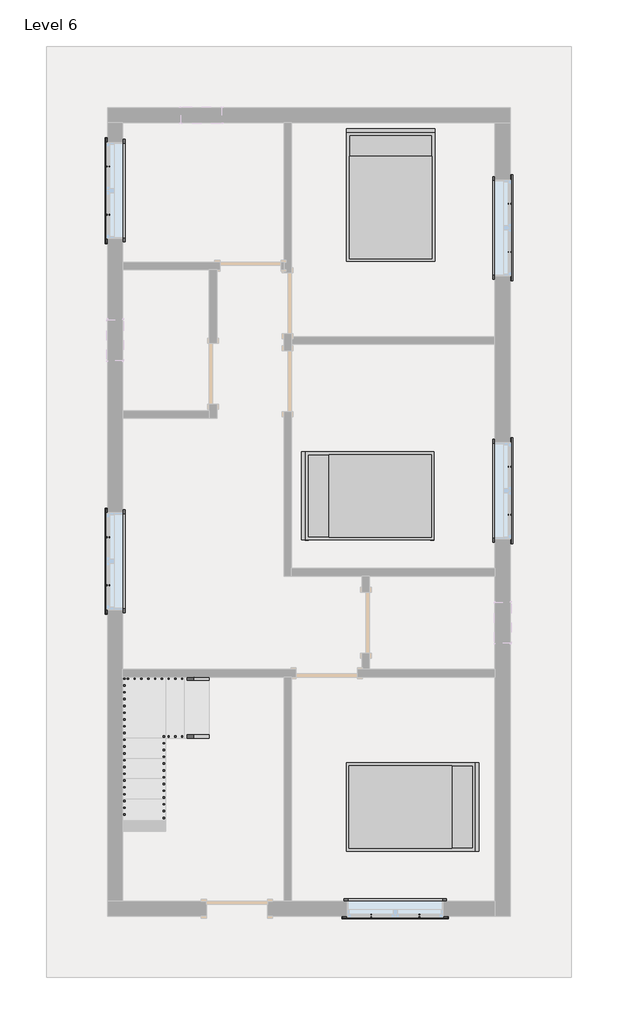
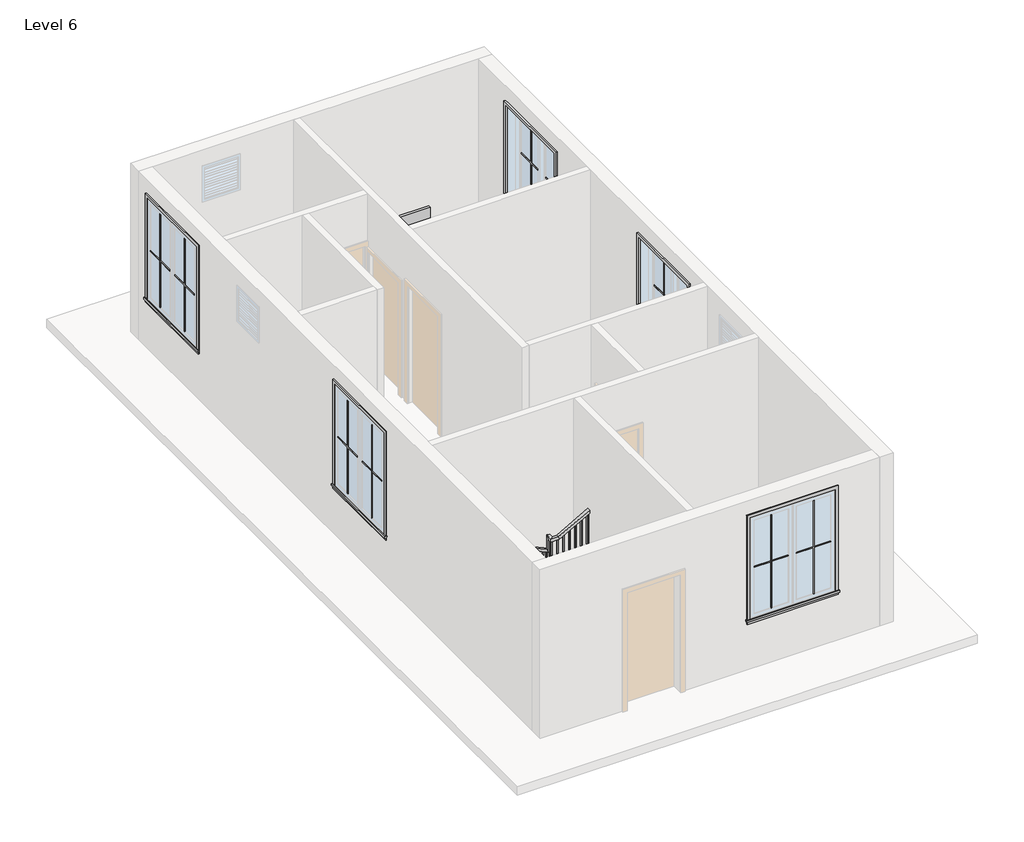
# One storey, part 2 of 2: 20 proxies, 3 furniture elements, 2 railings.
"""IFC4 building model written with IfcOpenShell, lengths in millimetres."""

from ifc_helpers import new_model, si_unit, frame, origin, place, context, project, spatial, polyline, outline, extrude, faceted_brep, transform, mapped, element, save
from components import muntin_pattern_2x2_muntin_pattern_2x2_bff912c5, muntin_pattern_2x2_muntin_pattern_2x2_c2194282, trim_window_exterior_flat_with_sill_e04b3088, trim_window_interior_flat_picture_frame_2a7685fe, bed_17739_bed_17739_15c61121

model = new_model("IFC4")

# Units and contexts
model_context = context("Model", 3, world=origin())
ifc_project = project(units=[si_unit("LENGTHUNIT", "METRE", prefix="MILLI")], contexts=[model_context])

# Site, building, storey
site = spatial("IfcSite", under=ifc_project)
building = spatial("IfcBuilding", under=site)
storey = spatial("IfcBuildingStorey", under=building, Name="Level 6", Elevation=12801.6)

# Proxies
placement = place(None, origin())
muntin_pattern_2x2_muntin_pattern_2x2_shape = muntin_pattern_2x2_muntin_pattern_2x2_bff912c5(model_context)
element("IfcBuildingElementProxy", 1, Name="Muntin Pattern_2x2 : Muntin Pattern_2x2", ObjectType="Muntin Pattern_2x2 : Muntin Pattern_2x2", at=placement, inside=storey, context=model_context, shape_type="MappedRepresentation", body=[
    mapped(muntin_pattern_2x2_muntin_pattern_2x2_shape, transform((-4261.9639285, 4584.2694249, 13785.85), x_axis=(0.0, 1.0, 0.0), y_axis=(-1.0, 0.0, 0.0), z_axis=(0.0, 0.0, 1.0))),
])
element("IfcBuildingElementProxy", 2, Name="Muntin Pattern_2x2 : Muntin Pattern_2x2", ObjectType="Muntin Pattern_2x2 : Muntin Pattern_2x2", at=placement, inside=storey, context=model_context, shape_type="MappedRepresentation", body=[
    mapped(muntin_pattern_2x2_muntin_pattern_2x2_shape, transform((1751.4860715, 4746.1944249, 13785.85), x_axis=(0.0, -1.0, 0.0), y_axis=(1.0, 0.0, 0.0), z_axis=(0.0, 0.0, 1.0))),
])
element("IfcBuildingElementProxy", 3, Name="Muntin Pattern_2x2 : Muntin Pattern_2x2", ObjectType="Muntin Pattern_2x2 : Muntin Pattern_2x2", at=placement, inside=storey, context=model_context, shape_type="MappedRepresentation", body=[
    mapped(muntin_pattern_2x2_muntin_pattern_2x2_shape, transform((-4261.9639285, -962.4555751, 13785.85), x_axis=(0.0, 1.0, 0.0), y_axis=(-1.0, 0.0, 0.0), z_axis=(0.0, 0.0, 1.0))),
])
element("IfcBuildingElementProxy", 4, Name="Muntin Pattern_2x2 : Muntin Pattern_2x2", ObjectType="Muntin Pattern_2x2 : Muntin Pattern_2x2", at=placement, inside=storey, context=model_context, shape_type="MappedRepresentation", body=[
    mapped(muntin_pattern_2x2_muntin_pattern_2x2_shape, transform((1751.4860715, 812.3694249, 13785.85), x_axis=(0.0, -1.0, 0.0), y_axis=(1.0, 0.0, 0.0), z_axis=(0.0, 0.0, 1.0))),
])
element("IfcBuildingElementProxy", 5, Name="Muntin Pattern_2x2 : Muntin Pattern_2x2", ObjectType="Muntin Pattern_2x2 : Muntin Pattern_2x2", at=placement, inside=storey, context=model_context, shape_type="MappedRepresentation", body=[
    mapped(muntin_pattern_2x2_muntin_pattern_2x2_shape, transform((397.3485715, -5907.5180751, 13785.85), x_axis=(-1.0, 0.0, 0.0), y_axis=(0.0, -1.0, 0.0), z_axis=(0.0, 0.0, 1.0))),
])
muntin_pattern_2x2_muntin_pattern_2x2_2_shape = muntin_pattern_2x2_muntin_pattern_2x2_c2194282(model_context)
element("IfcBuildingElementProxy", 6, Name="Muntin Pattern_2x2 : Muntin Pattern_2x2", ObjectType="Muntin Pattern_2x2 : Muntin Pattern_2x2", at=placement, inside=storey, context=model_context, shape_type="MappedRepresentation", body=[
    mapped(muntin_pattern_2x2_muntin_pattern_2x2_2_shape, transform((-4261.9639285, 5304.9944249, 13785.85), x_axis=(0.0, -1.0, 0.0), y_axis=(1.0, 0.0, 0.0), z_axis=(0.0, 0.0, 1.0))),
])
element("IfcBuildingElementProxy", 7, Name="Muntin Pattern_2x2 : Muntin Pattern_2x2", ObjectType="Muntin Pattern_2x2 : Muntin Pattern_2x2", at=placement, inside=storey, context=model_context, shape_type="MappedRepresentation", body=[
    mapped(muntin_pattern_2x2_muntin_pattern_2x2_2_shape, transform((1751.4860715, 4025.4694249, 13785.85), x_axis=(0.0, 1.0, 0.0), y_axis=(-1.0, 0.0, 0.0), z_axis=(0.0, 0.0, 1.0))),
])
element("IfcBuildingElementProxy", 8, Name="Muntin Pattern_2x2 : Muntin Pattern_2x2", ObjectType="Muntin Pattern_2x2 : Muntin Pattern_2x2", at=placement, inside=storey, context=model_context, shape_type="MappedRepresentation", body=[
    mapped(muntin_pattern_2x2_muntin_pattern_2x2_2_shape, transform((-4261.9639285, -241.7305751, 13785.85), x_axis=(0.0, -1.0, 0.0), y_axis=(1.0, 0.0, 0.0), z_axis=(0.0, 0.0, 1.0))),
])
element("IfcBuildingElementProxy", 9, Name="Muntin Pattern_2x2 : Muntin Pattern_2x2", ObjectType="Muntin Pattern_2x2 : Muntin Pattern_2x2", at=placement, inside=storey, context=model_context, shape_type="MappedRepresentation", body=[
    mapped(muntin_pattern_2x2_muntin_pattern_2x2_2_shape, transform((1751.4860715, 91.6444249, 13785.85), x_axis=(0.0, 1.0, 0.0), y_axis=(-1.0, 0.0, 0.0), z_axis=(0.0, 0.0, 1.0))),
])
element("IfcBuildingElementProxy", 10, Name="Muntin Pattern_2x2 : Muntin Pattern_2x2", ObjectType="Muntin Pattern_2x2 : Muntin Pattern_2x2", at=placement, inside=storey, context=model_context, shape_type="MappedRepresentation", body=[
    mapped(muntin_pattern_2x2_muntin_pattern_2x2_2_shape, transform((-323.3764285, -5907.5180751, 13785.85), x_axis=(1.0, 0.0, 0.0), y_axis=(0.0, 1.0, 0.0), z_axis=(0.0, 0.0, 1.0))),
])
trim_window_exterior_flat_with_sill_shape = trim_window_exterior_flat_with_sill_e04b3088(model_context)
element("IfcBuildingElementProxy", 11, Name="Trim-Window-Exterior-Flat : with Sill", ObjectType="Trim-Window-Exterior-Flat : with Sill", at=placement, inside=storey, context=model_context, shape_type="MappedRepresentation", body=[
    mapped(trim_window_exterior_flat_with_sill_shape, transform((-4271.4889285, 4944.6319249, 15544.8), x_axis=(0.0, -1.0, 0.0), y_axis=(0.0, 0.0, 1.0), z_axis=(-1.0, 0.0, 0.0))),
])
element("IfcBuildingElementProxy", 12, Name="Trim-Window-Exterior-Flat : with Sill", ObjectType="Trim-Window-Exterior-Flat : with Sill", at=placement, inside=storey, context=model_context, shape_type="MappedRepresentation", body=[
    mapped(trim_window_exterior_flat_with_sill_shape, transform((1761.0110715, 4385.8319249, 15544.8), x_axis=(0.0, 1.0, 0.0), y_axis=(0.0, 0.0, 1.0), z_axis=(1.0, 0.0, 0.0))),
])
element("IfcBuildingElementProxy", 13, Name="Trim-Window-Exterior-Flat : with Sill", ObjectType="Trim-Window-Exterior-Flat : with Sill", at=placement, inside=storey, context=model_context, shape_type="MappedRepresentation", body=[
    mapped(trim_window_exterior_flat_with_sill_shape, transform((-4271.4889285, -602.0930751, 15544.8), x_axis=(0.0, -1.0, 0.0), y_axis=(0.0, 0.0, 1.0), z_axis=(-1.0, 0.0, 0.0))),
])
element("IfcBuildingElementProxy", 14, Name="Trim-Window-Exterior-Flat : with Sill", ObjectType="Trim-Window-Exterior-Flat : with Sill", at=placement, inside=storey, context=model_context, shape_type="MappedRepresentation", body=[
    mapped(trim_window_exterior_flat_with_sill_shape, transform((1761.0110715, 452.0069249, 15544.8), x_axis=(0.0, 1.0, 0.0), y_axis=(0.0, 0.0, 1.0), z_axis=(1.0, 0.0, 0.0))),
])
element("IfcBuildingElementProxy", 15, Name="Trim-Window-Exterior-Flat : with Sill", ObjectType="Trim-Window-Exterior-Flat : with Sill", at=placement, inside=storey, context=model_context, shape_type="MappedRepresentation", body=[
    mapped(trim_window_exterior_flat_with_sill_shape, transform((36.9860715, -5917.0430751, 15544.8), x_axis=(1.0, 0.0, 0.0), y_axis=(0.0, 0.0, 1.0), z_axis=(0.0, -1.0, 0.0))),
])
trim_window_interior_flat_picture_frame_shape = trim_window_interior_flat_picture_frame_2a7685fe(model_context)
element("IfcBuildingElementProxy", 16, Name="Trim-Window-Interior-Flat : Picture Frame", ObjectType="Trim-Window-Interior-Flat : Picture Frame", at=placement, inside=storey, context=model_context, shape_type="MappedRepresentation", body=[
    mapped(trim_window_interior_flat_picture_frame_shape, transform((-4042.8889285, 4944.6319249, 15544.8), x_axis=(0.0, 1.0, 0.0), y_axis=(0.0, 0.0, 1.0), z_axis=(1.0, 0.0, 0.0))),
])
element("IfcBuildingElementProxy", 17, Name="Trim-Window-Interior-Flat : Picture Frame", ObjectType="Trim-Window-Interior-Flat : Picture Frame", at=placement, inside=storey, context=model_context, shape_type="MappedRepresentation", body=[
    mapped(trim_window_interior_flat_picture_frame_shape, transform((1532.4110715, 4385.8319249, 15544.8), x_axis=(0.0, -1.0, 0.0), y_axis=(0.0, 0.0, 1.0), z_axis=(-1.0, 0.0, 0.0))),
])
element("IfcBuildingElementProxy", 18, Name="Trim-Window-Interior-Flat : Picture Frame", ObjectType="Trim-Window-Interior-Flat : Picture Frame", at=placement, inside=storey, context=model_context, shape_type="MappedRepresentation", body=[
    mapped(trim_window_interior_flat_picture_frame_shape, transform((-4042.8889285, -602.0930751, 15544.8), x_axis=(0.0, 1.0, 0.0), y_axis=(0.0, 0.0, 1.0), z_axis=(1.0, 0.0, 0.0))),
])
element("IfcBuildingElementProxy", 19, Name="Trim-Window-Interior-Flat : Picture Frame", ObjectType="Trim-Window-Interior-Flat : Picture Frame", at=placement, inside=storey, context=model_context, shape_type="MappedRepresentation", body=[
    mapped(trim_window_interior_flat_picture_frame_shape, transform((1532.4110715, 452.0069249, 15544.8), x_axis=(0.0, -1.0, 0.0), y_axis=(0.0, 0.0, 1.0), z_axis=(-1.0, 0.0, 0.0))),
])
element("IfcBuildingElementProxy", 20, Name="Trim-Window-Interior-Flat : Picture Frame", ObjectType="Trim-Window-Interior-Flat : Picture Frame", at=placement, inside=storey, context=model_context, shape_type="MappedRepresentation", body=[
    mapped(trim_window_interior_flat_picture_frame_shape, transform((36.9860715, -5688.4430751, 15544.8), x_axis=(-1.0, 0.0, 0.0), y_axis=(0.0, 0.0, 1.0), z_axis=(0.0, 1.0, 0.0))),
])

# Furniture
bed_17739_bed_17739_shape = bed_17739_bed_17739_15c61121(model_context)
element("IfcFurniture", 21, ObjectType="Bed_17739 : Bed_17739", at=placement, inside=storey, context=model_context, shape_type="MappedRepresentation", body=[
    mapped(bed_17739_bed_17739_shape, transform((-29.6889285, 4852.5569249, 12801.6), x_axis=(1.0, 0.0, 0.0), y_axis=(0.0, 1.0, 0.0), z_axis=(0.0, 0.0, 1.0))),
])
element("IfcFurniture", 22, ObjectType="Bed_17739 : Bed_17739", at=placement, inside=storey, context=model_context, shape_type="MappedRepresentation", body=[
    mapped(bed_17739_bed_17739_shape, transform((-347.1889285, 375.8069249, 12801.6), x_axis=(0.0, 1.0, 0.0), y_axis=(-1.0, 0.0, 0.0), z_axis=(0.0, 0.0, 1.0))),
])
element("IfcFurniture", 23, ObjectType="Bed_17739 : Bed_17739", at=placement, inside=storey, context=model_context, shape_type="MappedRepresentation", body=[
    mapped(bed_17739_bed_17739_shape, transform((275.1110715, -4278.7430751, 12801.6), x_axis=(0.0, -1.0, 0.0), y_axis=(1.0, 0.0, 0.0), z_axis=(0.0, 0.0, 1.0))),
])

# Railings
element("IfcRailing", 24, ObjectType="Handrail - Rectangular", at=placement, inside=storey, context=model_context, shape_type="SolidModel", body=[
    faceted_brep([(-2747.4889285, -2386.4430751, 13885.3333333), (-2747.4889285, -2386.4430751, 13828.1271159), (-2747.4889285, -2335.6430751, 13828.1271159), (-2747.4889285, -2335.6430751, 13885.3333333), (-3396.0267484, -2386.4430751, 14221.1457967), (-3408.3987558, -2386.4430751, 14170.3457967), (-3408.3987558, -2335.6430751, 14170.3457967), (-3396.0267484, -2335.6430751, 14221.1457967), (-3992.0889285, -2386.4430751, 14221.1457967), (-3992.0889285, -2386.4430751, 14170.3457967), (-4042.8889285, -2335.6430751, 14170.3457967), (-4042.8889285, -2335.6430751, 14221.1457967), (-3992.0889285, -2940.1628326, 14221.1457967), (-3992.0889285, -2953.3285634, 14170.3457967), (-4042.8889285, -2953.3285634, 14170.3457967), (-4042.8889285, -2940.1628326, 14221.1457967), (-3992.0889285, -5061.9991591, 15400.1618165), (-3992.0889285, -5075.1648899, 15349.3618165), (-4042.8889285, -5075.1648899, 15349.3618165), (-4042.8889285, -5061.9991591, 15400.1618165), (-3992.0889285, -5637.6430751, 15400.1618165), (-3992.0889285, -5637.6430751, 15349.3618165), (-4042.8889285, -5688.4430751, 15349.3618165), (-4042.8889285, -5688.4430751, 15400.1618165), (-3418.001852, -5637.6430751, 15400.1618165), (-3404.8062484, -5637.6430751, 15349.3618165), (-3404.8062484, -5688.4430751, 15349.3618165), (-3418.001852, -5688.4430751, 15400.1618165), (-2793.6303845, -5637.6430751, 15748.0), (-2793.6303845, -5688.4430751, 15748.0), (-2793.6303845, -5688.4430751, 15689.8487115), (-2793.6303845, -5637.6430751, 15689.8487115)], [[[0, 1, 2, 3]], [[1, 0, 4, 5]], [[2, 1, 5, 6]], [[3, 2, 6, 7]], [[0, 3, 7, 4]], [[5, 4, 8, 9]], [[6, 5, 9, 10]], [[7, 6, 10, 11]], [[4, 7, 11, 8]], [[9, 8, 12, 13]], [[10, 9, 13, 14]], [[11, 10, 14, 15]], [[8, 11, 15, 12]], [[13, 12, 16, 17]], [[14, 13, 17, 18]], [[15, 14, 18, 19]], [[12, 15, 19, 16]], [[17, 16, 20, 21]], [[18, 17, 21, 22]], [[19, 18, 22, 23]], [[16, 19, 23, 20]], [[21, 20, 24, 25]], [[22, 21, 25, 26]], [[23, 22, 26, 27]], [[20, 23, 27, 24]], [[28, 29, 30, 31]], [[25, 24, 28, 31]], [[26, 25, 31, 30]], [[27, 26, 30, 29]], [[24, 27, 29, 28]]]),
    extrude(outline(polyline([(15692.5598207, -2788.7639285), (15681.9470401, -2807.8139285), (14664.2666667, -2807.8139285), (14664.2666667, -2788.7639285), (15692.5598207, -2788.7639285)])), frame((0.0, -5672.5680751, 0.0), z_axis=(0.0, 1.0, 0.0), x_axis=(0.0, 0.0, 1.0)), (0.0, 0.0, 1.0), 19.05),
    extrude(outline(polyline([(15635.9583242, -2890.3639285), (15625.3455436, -2909.4139285), (14664.2666667, -2909.4139285), (14664.2666667, -2890.3639285), (15635.9583242, -2890.3639285)])), frame((0.0, -5672.5680751, 0.0), z_axis=(0.0, 1.0, 0.0), x_axis=(0.0, 0.0, 1.0)), (0.0, 0.0, 1.0), 19.05),
    extrude(outline(polyline([(15579.3568277, -2991.9639285), (15568.7440471, -3011.0139285), (14664.2666667, -3011.0139285), (14664.2666667, -2991.9639285), (15579.3568277, -2991.9639285)])), frame((0.0, -5672.5680751, 0.0), z_axis=(0.0, 1.0, 0.0), x_axis=(0.0, 0.0, 1.0)), (0.0, 0.0, 1.0), 19.05),
    extrude(outline(polyline([(15522.7553312, -3093.5639285), (15512.1425506, -3112.6139285), (14664.2666667, -3112.6139285), (14664.2666667, -3093.5639285), (15522.7553312, -3093.5639285)])), frame((0.0, -5672.5680751, 0.0), z_axis=(0.0, 1.0, 0.0), x_axis=(0.0, 0.0, 1.0)), (0.0, 0.0, 1.0), 19.05),
    extrude(outline(polyline([(15466.1538346, -3195.1639285), (15455.5410541, -3214.2139285), (14494.9333333, -3214.2139285), (14494.9333333, -3195.1639285), (15466.1538346, -3195.1639285)])), frame((0.0, -5672.5680751, 0.0), z_axis=(0.0, 1.0, 0.0), x_axis=(0.0, 0.0, 1.0)), (0.0, 0.0, 1.0), 19.05),
    extrude(outline(polyline([(15409.5523381, -3296.7639285), (15398.9395575, -3315.8139285), (14494.9333333, -3315.8139285), (14494.9333333, -3296.7639285), (15409.5523381, -3296.7639285)])), frame((0.0, -5672.5680751, 0.0), z_axis=(0.0, 1.0, 0.0), x_axis=(0.0, 0.0, 1.0)), (0.0, 0.0, 1.0), 19.05),
    extrude(outline(polyline([(15352.9508416, -3398.3639285), (15342.338061, -3417.4139285), (14325.6, -3417.4139285), (14325.6, -3398.3639285), (15352.9508416, -3398.3639285)])), frame((0.0, -5672.5680751, 0.0), z_axis=(0.0, 1.0, 0.0), x_axis=(0.0, 0.0, 1.0)), (0.0, 0.0, 1.0), 19.05),
    extrude(outline(polyline([(-3519.0139285, -5672.5680751), (-3519.0139285, -5653.5180751), (-3499.9639285, -5653.5180751), (-3499.9639285, -5672.5680751), (-3519.0139285, -5672.5680751)])), frame((0.0, 0.0, 14325.6), z_axis=(0.0, 0.0, 1.0), x_axis=(1.0, 0.0, 0.0)), (0.0, 0.0, 1.0), 1023.7618165),
    extrude(outline(polyline([(-3620.6139285, -5672.5680751), (-3620.6139285, -5653.5180751), (-3601.5639285, -5653.5180751), (-3601.5639285, -5672.5680751), (-3620.6139285, -5672.5680751)])), frame((0.0, 0.0, 14325.6), z_axis=(0.0, 0.0, 1.0), x_axis=(1.0, 0.0, 0.0)), (0.0, 0.0, 1.0), 1023.7618165),
    extrude(outline(polyline([(-3722.2139285, -5672.5680751), (-3722.2139285, -5653.5180751), (-3703.1639285, -5653.5180751), (-3703.1639285, -5672.5680751), (-3722.2139285, -5672.5680751)])), frame((0.0, 0.0, 14325.6), z_axis=(0.0, 0.0, 1.0), x_axis=(1.0, 0.0, 0.0)), (0.0, 0.0, 1.0), 1023.7618165),
    extrude(outline(polyline([(-3823.8139285, -5672.5680751), (-3823.8139285, -5653.5180751), (-3804.7639285, -5653.5180751), (-3804.7639285, -5672.5680751), (-3823.8139285, -5672.5680751)])), frame((0.0, 0.0, 14325.6), z_axis=(0.0, 0.0, 1.0), x_axis=(1.0, 0.0, 0.0)), (0.0, 0.0, 1.0), 1023.7618165),
    extrude(outline(polyline([(-3925.4139285, -5672.5680751), (-3925.4139285, -5653.5180751), (-3906.3639285, -5653.5180751), (-3906.3639285, -5672.5680751), (-3925.4139285, -5672.5680751)])), frame((0.0, 0.0, 14325.6), z_axis=(0.0, 0.0, 1.0), x_axis=(1.0, 0.0, 0.0)), (0.0, 0.0, 1.0), 1023.7618165),
    extrude(outline(polyline([(-4027.0139285, -5602.7180751), (-4007.9639285, -5602.7180751), (-4007.9639285, -5621.7680751), (-4027.0139285, -5621.7680751), (-4027.0139285, -5602.7180751)])), frame((0.0, 0.0, 14325.6), z_axis=(0.0, 0.0, 1.0), x_axis=(1.0, 0.0, 0.0)), (0.0, 0.0, 1.0), 1023.7618165),
    extrude(outline(polyline([(-4027.0139285, -5501.1180751), (-4007.9639285, -5501.1180751), (-4007.9639285, -5520.1680751), (-4027.0139285, -5520.1680751), (-4027.0139285, -5501.1180751)])), frame((0.0, 0.0, 14325.6), z_axis=(0.0, 0.0, 1.0), x_axis=(1.0, 0.0, 0.0)), (0.0, 0.0, 1.0), 1023.7618165),
    extrude(outline(polyline([(-4027.0139285, -5399.5180751), (-4007.9639285, -5399.5180751), (-4007.9639285, -5418.5680751), (-4027.0139285, -5418.5680751), (-4027.0139285, -5399.5180751)])), frame((0.0, 0.0, 14325.6), z_axis=(0.0, 0.0, 1.0), x_axis=(1.0, 0.0, 0.0)), (0.0, 0.0, 1.0), 1023.7618165),
    extrude(outline(polyline([(-4027.0139285, -5297.9180751), (-4007.9639285, -5297.9180751), (-4007.9639285, -5316.9680751), (-4027.0139285, -5316.9680751), (-4027.0139285, -5297.9180751)])), frame((0.0, 0.0, 14325.6), z_axis=(0.0, 0.0, 1.0), x_axis=(1.0, 0.0, 0.0)), (0.0, 0.0, 1.0), 1023.7618165),
    extrude(outline(polyline([(-4027.0139285, -5196.3180751), (-4007.9639285, -5196.3180751), (-4007.9639285, -5215.3680751), (-4027.0139285, -5215.3680751), (-4027.0139285, -5196.3180751)])), frame((0.0, 0.0, 14325.6), z_axis=(0.0, 0.0, 1.0), x_axis=(1.0, 0.0, 0.0)), (0.0, 0.0, 1.0), 1023.7618165),
    extrude(outline(polyline([(-4027.0139285, -5094.7180751), (-4007.9639285, -5094.7180751), (-4007.9639285, -5113.7680751), (-4027.0139285, -5113.7680751), (-4027.0139285, -5094.7180751)])), frame((0.0, 0.0, 14325.6), z_axis=(0.0, 0.0, 1.0), x_axis=(1.0, 0.0, 0.0)), (0.0, 0.0, 1.0), 1023.7618165),
    extrude(outline(polyline([(-5012.1680751, 15314.3571119), (-4993.1180751, 15303.7718208), (-4993.1180751, 14325.6), (-5012.1680751, 14325.6), (-5012.1680751, 15314.3571119)])), frame((-4027.0139285, 0.0, 0.0), z_axis=(1.0, 0.0, 0.0), x_axis=(0.0, 1.0, 0.0)), (0.0, 0.0, 1.0), 19.05),
    extrude(outline(polyline([(-4910.5680751, 15257.9022261), (-4891.5180751, 15247.316935), (-4891.5180751, 14325.6), (-4910.5680751, 14325.6), (-4910.5680751, 15257.9022261)])), frame((-4027.0139285, 0.0, 0.0), z_axis=(1.0, 0.0, 0.0), x_axis=(0.0, 1.0, 0.0)), (0.0, 0.0, 1.0), 19.05),
    extrude(outline(polyline([(-4808.9680751, 15201.4473402), (-4789.9180751, 15190.8620491), (-4789.9180751, 14325.6), (-4808.9680751, 14325.6), (-4808.9680751, 15201.4473402)])), frame((-4027.0139285, 0.0, 0.0), z_axis=(1.0, 0.0, 0.0), x_axis=(0.0, 1.0, 0.0)), (0.0, 0.0, 1.0), 19.05),
    extrude(outline(polyline([(-4707.3680751, 15144.8358332), (-4688.3180751, 15134.2505421), (-4688.3180751, 14156.2666667), (-4707.3680751, 14156.2666667), (-4707.3680751, 15144.8358332)])), frame((-4027.0139285, 0.0, 0.0), z_axis=(1.0, 0.0, 0.0), x_axis=(0.0, 1.0, 0.0)), (0.0, 0.0, 1.0), 19.05),
    extrude(outline(polyline([(-4605.7680751, 15088.3809474), (-4586.7180751, 15077.7956563), (-4586.7180751, 14156.2666667), (-4605.7680751, 14156.2666667), (-4605.7680751, 15088.3809474)])), frame((-4027.0139285, 0.0, 0.0), z_axis=(1.0, 0.0, 0.0), x_axis=(0.0, 1.0, 0.0)), (0.0, 0.0, 1.0), 19.05),
    extrude(outline(polyline([(-4504.1680751, 15031.9260615), (-4485.1180751, 15021.3407704), (-4485.1180751, 14156.2666667), (-4504.1680751, 14156.2666667), (-4504.1680751, 15031.9260615)])), frame((-4027.0139285, 0.0, 0.0), z_axis=(1.0, 0.0, 0.0), x_axis=(0.0, 1.0, 0.0)), (0.0, 0.0, 1.0), 19.05),
    extrude(outline(polyline([(-4402.5680751, 14975.5024999), (-4383.5180751, 14964.9172088), (-4383.5180751, 13986.9333333), (-4402.5680751, 13986.9333333), (-4402.5680751, 14975.5024999)])), frame((-4027.0139285, 0.0, 0.0), z_axis=(1.0, 0.0, 0.0), x_axis=(0.0, 1.0, 0.0)), (0.0, 0.0, 1.0), 19.05),
    extrude(outline(polyline([(-4300.9680751, 14919.047614), (-4281.9180751, 14908.4623229), (-4281.9180751, 13986.9333333), (-4300.9680751, 13986.9333333), (-4300.9680751, 14919.047614)])), frame((-4027.0139285, 0.0, 0.0), z_axis=(1.0, 0.0, 0.0), x_axis=(0.0, 1.0, 0.0)), (0.0, 0.0, 1.0), 19.05),
    extrude(outline(polyline([(-4199.3680751, 14862.5927282), (-4180.3180751, 14852.0074371), (-4180.3180751, 13986.9333333), (-4199.3680751, 13986.9333333), (-4199.3680751, 14862.5927282)])), frame((-4027.0139285, 0.0, 0.0), z_axis=(1.0, 0.0, 0.0), x_axis=(0.0, 1.0, 0.0)), (0.0, 0.0, 1.0), 19.05),
    extrude(outline(polyline([(-4097.7680751, 14806.1691666), (-4078.7180751, 14795.5838755), (-4078.7180751, 13817.6), (-4097.7680751, 13817.6), (-4097.7680751, 14806.1691666)])), frame((-4027.0139285, 0.0, 0.0), z_axis=(1.0, 0.0, 0.0), x_axis=(0.0, 1.0, 0.0)), (0.0, 0.0, 1.0), 19.05),
    extrude(outline(polyline([(-3996.1680751, 14749.7142807), (-3977.1180751, 14739.1289896), (-3977.1180751, 13817.6), (-3996.1680751, 13817.6), (-3996.1680751, 14749.7142807)])), frame((-4027.0139285, 0.0, 0.0), z_axis=(1.0, 0.0, 0.0), x_axis=(0.0, 1.0, 0.0)), (0.0, 0.0, 1.0), 19.05),
    extrude(outline(polyline([(-3894.5680751, 14693.2593949), (-3875.5180751, 14682.6741038), (-3875.5180751, 13817.6), (-3894.5680751, 13817.6), (-3894.5680751, 14693.2593949)])), frame((-4027.0139285, 0.0, 0.0), z_axis=(1.0, 0.0, 0.0), x_axis=(0.0, 1.0, 0.0)), (0.0, 0.0, 1.0), 19.05),
    extrude(outline(polyline([(-3792.9680751, 14636.8358332), (-3773.9180751, 14626.2505421), (-3773.9180751, 13648.2666667), (-3792.9680751, 13648.2666667), (-3792.9680751, 14636.8358332)])), frame((-4027.0139285, 0.0, 0.0), z_axis=(1.0, 0.0, 0.0), x_axis=(0.0, 1.0, 0.0)), (0.0, 0.0, 1.0), 19.05),
    extrude(outline(polyline([(-3691.3680751, 14580.3809474), (-3672.3180751, 14569.7956563), (-3672.3180751, 13648.2666667), (-3691.3680751, 13648.2666667), (-3691.3680751, 14580.3809474)])), frame((-4027.0139285, 0.0, 0.0), z_axis=(1.0, 0.0, 0.0), x_axis=(0.0, 1.0, 0.0)), (0.0, 0.0, 1.0), 19.05),
    extrude(outline(polyline([(-3589.7680751, 14523.9260615), (-3570.7180751, 14513.3407704), (-3570.7180751, 13648.2666667), (-3589.7680751, 13648.2666667), (-3589.7680751, 14523.9260615)])), frame((-4027.0139285, 0.0, 0.0), z_axis=(1.0, 0.0, 0.0), x_axis=(0.0, 1.0, 0.0)), (0.0, 0.0, 1.0), 19.05),
    extrude(outline(polyline([(-3488.1680751, 14467.5024999), (-3469.1180751, 14456.9172088), (-3469.1180751, 13478.9333333), (-3488.1680751, 13478.9333333), (-3488.1680751, 14467.5024999)])), frame((-4027.0139285, 0.0, 0.0), z_axis=(1.0, 0.0, 0.0), x_axis=(0.0, 1.0, 0.0)), (0.0, 0.0, 1.0), 19.05),
    extrude(outline(polyline([(-3386.5680751, 14411.047614), (-3367.5180751, 14400.4623229), (-3367.5180751, 13478.9333333), (-3386.5680751, 13478.9333333), (-3386.5680751, 14411.047614)])), frame((-4027.0139285, 0.0, 0.0), z_axis=(1.0, 0.0, 0.0), x_axis=(0.0, 1.0, 0.0)), (0.0, 0.0, 1.0), 19.05),
    extrude(outline(polyline([(-3284.9680751, 14354.5927282), (-3265.9180751, 14344.0074371), (-3265.9180751, 13478.9333333), (-3284.9680751, 13478.9333333), (-3284.9680751, 14354.5927282)])), frame((-4027.0139285, 0.0, 0.0), z_axis=(1.0, 0.0, 0.0), x_axis=(0.0, 1.0, 0.0)), (0.0, 0.0, 1.0), 19.05),
    extrude(outline(polyline([(-3183.3680751, 14298.1691666), (-3164.3180751, 14287.5838755), (-3164.3180751, 13309.6), (-3183.3680751, 13309.6), (-3183.3680751, 14298.1691666)])), frame((-4027.0139285, 0.0, 0.0), z_axis=(1.0, 0.0, 0.0), x_axis=(0.0, 1.0, 0.0)), (0.0, 0.0, 1.0), 19.05),
    extrude(outline(polyline([(-3081.7680751, 14241.7142807), (-3062.7180751, 14231.1289896), (-3062.7180751, 13309.6), (-3081.7680751, 13309.6), (-3081.7680751, 14241.7142807)])), frame((-4027.0139285, 0.0, 0.0), z_axis=(1.0, 0.0, 0.0), x_axis=(0.0, 1.0, 0.0)), (0.0, 0.0, 1.0), 19.05),
    extrude(outline(polyline([(-2980.1680751, 14185.2593949), (-2961.1180751, 14174.6741038), (-2961.1180751, 13309.6), (-2980.1680751, 13309.6), (-2980.1680751, 14185.2593949)])), frame((-4027.0139285, 0.0, 0.0), z_axis=(1.0, 0.0, 0.0), x_axis=(0.0, 1.0, 0.0)), (0.0, 0.0, 1.0), 19.05),
    extrude(outline(polyline([(-4027.0139285, -2859.5180751), (-4007.9639285, -2859.5180751), (-4007.9639285, -2878.5680751), (-4027.0139285, -2878.5680751), (-4027.0139285, -2859.5180751)])), frame((0.0, 0.0, 13309.6), z_axis=(0.0, 0.0, 1.0), x_axis=(1.0, 0.0, 0.0)), (0.0, 0.0, 1.0), 860.7457967),
    extrude(outline(polyline([(-4027.0139285, -2757.9180751), (-4007.9639285, -2757.9180751), (-4007.9639285, -2776.9680751), (-4027.0139285, -2776.9680751), (-4027.0139285, -2757.9180751)])), frame((0.0, 0.0, 13309.6), z_axis=(0.0, 0.0, 1.0), x_axis=(1.0, 0.0, 0.0)), (0.0, 0.0, 1.0), 860.7457967),
    extrude(outline(polyline([(-4027.0139285, -2656.3180751), (-4007.9639285, -2656.3180751), (-4007.9639285, -2675.3680751), (-4027.0139285, -2675.3680751), (-4027.0139285, -2656.3180751)])), frame((0.0, 0.0, 13309.6), z_axis=(0.0, 0.0, 1.0), x_axis=(1.0, 0.0, 0.0)), (0.0, 0.0, 1.0), 860.7457967),
    extrude(outline(polyline([(-4027.0139285, -2554.7180751), (-4007.9639285, -2554.7180751), (-4007.9639285, -2573.7680751), (-4027.0139285, -2573.7680751), (-4027.0139285, -2554.7180751)])), frame((0.0, 0.0, 13309.6), z_axis=(0.0, 0.0, 1.0), x_axis=(1.0, 0.0, 0.0)), (0.0, 0.0, 1.0), 860.7457967),
    extrude(outline(polyline([(-4027.0139285, -2453.1180751), (-4007.9639285, -2453.1180751), (-4007.9639285, -2472.1680751), (-4027.0139285, -2472.1680751), (-4027.0139285, -2453.1180751)])), frame((0.0, 0.0, 13309.6), z_axis=(0.0, 0.0, 1.0), x_axis=(1.0, 0.0, 0.0)), (0.0, 0.0, 1.0), 860.7457967),
    extrude(outline(polyline([(-3957.1639285, -2351.5180751), (-3957.1639285, -2370.5680751), (-3976.2139285, -2370.5680751), (-3976.2139285, -2351.5180751), (-3957.1639285, -2351.5180751)])), frame((0.0, 0.0, 13309.6), z_axis=(0.0, 0.0, 1.0), x_axis=(1.0, 0.0, 0.0)), (0.0, 0.0, 1.0), 860.7457967),
    extrude(outline(polyline([(-3855.5639285, -2351.5180751), (-3855.5639285, -2370.5680751), (-3874.6139285, -2370.5680751), (-3874.6139285, -2351.5180751), (-3855.5639285, -2351.5180751)])), frame((0.0, 0.0, 13309.6), z_axis=(0.0, 0.0, 1.0), x_axis=(1.0, 0.0, 0.0)), (0.0, 0.0, 1.0), 860.7457967),
    extrude(outline(polyline([(-3753.9639285, -2351.5180751), (-3753.9639285, -2370.5680751), (-3773.0139285, -2370.5680751), (-3773.0139285, -2351.5180751), (-3753.9639285, -2351.5180751)])), frame((0.0, 0.0, 13309.6), z_axis=(0.0, 0.0, 1.0), x_axis=(1.0, 0.0, 0.0)), (0.0, 0.0, 1.0), 860.7457967),
    extrude(outline(polyline([(-3652.3639285, -2351.5180751), (-3652.3639285, -2370.5680751), (-3671.4139285, -2370.5680751), (-3671.4139285, -2351.5180751), (-3652.3639285, -2351.5180751)])), frame((0.0, 0.0, 13309.6), z_axis=(0.0, 0.0, 1.0), x_axis=(1.0, 0.0, 0.0)), (0.0, 0.0, 1.0), 860.7457967),
    extrude(outline(polyline([(-3550.7639285, -2351.5180751), (-3550.7639285, -2370.5680751), (-3569.8139285, -2370.5680751), (-3569.8139285, -2351.5180751), (-3550.7639285, -2351.5180751)])), frame((0.0, 0.0, 13309.6), z_axis=(0.0, 0.0, 1.0), x_axis=(1.0, 0.0, 0.0)), (0.0, 0.0, 1.0), 860.7457967),
    extrude(outline(polyline([(-3449.1639285, -2351.5180751), (-3449.1639285, -2370.5680751), (-3468.2139285, -2370.5680751), (-3468.2139285, -2351.5180751), (-3449.1639285, -2351.5180751)])), frame((0.0, 0.0, 13309.6), z_axis=(0.0, 0.0, 1.0), x_axis=(1.0, 0.0, 0.0)), (0.0, 0.0, 1.0), 860.7457967),
    extrude(outline(polyline([(14138.8455625, -3347.5639285), (14148.7096402, -3366.6139285), (13140.2666667, -3366.6139285), (13140.2666667, -3347.5639285), (14138.8455625, -3347.5639285)])), frame((0.0, -2370.5680751, 0.0), z_axis=(0.0, 1.0, 0.0), x_axis=(0.0, 0.0, 1.0)), (0.0, 0.0, 1.0), 19.05),
    extrude(outline(polyline([(14086.2371483, -3245.9639285), (14096.1012259, -3265.0139285), (13140.2666667, -3265.0139285), (13140.2666667, -3245.9639285), (14086.2371483, -3245.9639285)])), frame((0.0, -2370.5680751, 0.0), z_axis=(0.0, 1.0, 0.0), x_axis=(0.0, 0.0, 1.0)), (0.0, 0.0, 1.0), 19.05),
    extrude(outline(polyline([(14033.628734, -3144.3639285), (14043.4928117, -3163.4139285), (13140.2666667, -3163.4139285), (13140.2666667, -3144.3639285), (14033.628734, -3144.3639285)])), frame((0.0, -2370.5680751, 0.0), z_axis=(0.0, 1.0, 0.0), x_axis=(0.0, 0.0, 1.0)), (0.0, 0.0, 1.0), 19.05),
    extrude(outline(polyline([(13981.0203198, -3042.7639285), (13990.8843975, -3061.8139285), (12970.9333333, -3061.8139285), (12970.9333333, -3042.7639285), (13981.0203198, -3042.7639285)])), frame((0.0, -2370.5680751, 0.0), z_axis=(0.0, 1.0, 0.0), x_axis=(0.0, 0.0, 1.0)), (0.0, 0.0, 1.0), 19.05),
    extrude(outline(polyline([(13928.4119056, -2941.1639285), (13938.2759832, -2960.2139285), (12970.9333333, -2960.2139285), (12970.9333333, -2941.1639285), (13928.4119056, -2941.1639285)])), frame((0.0, -2370.5680751, 0.0), z_axis=(0.0, 1.0, 0.0), x_axis=(0.0, 0.0, 1.0)), (0.0, 0.0, 1.0), 19.05),
    extrude(outline(polyline([(13875.8034913, -2839.5639285), (13885.667569, -2858.6139285), (12970.9333333, -2858.6139285), (12970.9333333, -2839.5639285), (13875.8034913, -2839.5639285)])), frame((0.0, -2370.5680751, 0.0), z_axis=(0.0, 1.0, 0.0), x_axis=(0.0, 0.0, 1.0)), (0.0, 0.0, 1.0), 19.05),
    extrude(outline(polyline([(-4027.0139285, -5653.5180751), (-4007.9639285, -5653.5180751), (-4007.9639285, -5672.5680751), (-4027.0139285, -5672.5680751), (-4027.0139285, -5653.5180751)])), frame((0.0, 0.0, 14325.6), z_axis=(0.0, 0.0, 1.0), x_axis=(1.0, 0.0, 0.0)), (0.0, 0.0, 1.0), 1023.7618165),
    extrude(outline(polyline([(-4007.9639285, -2351.5180751), (-4007.9639285, -2370.5680751), (-4027.0139285, -2370.5680751), (-4027.0139285, -2351.5180751), (-4007.9639285, -2351.5180751)])), frame((0.0, 0.0, 13309.6), z_axis=(0.0, 0.0, 1.0), x_axis=(1.0, 0.0, 0.0)), (0.0, 0.0, 1.0), 860.7457967),
    extrude(outline(polyline([(15689.8487115, -2793.6303845), (15679.2359309, -2812.6803845), (14664.2666667, -2812.6803845), (14664.2666667, -2793.6303845), (15689.8487115, -2793.6303845)])), frame((0.0, -5672.5680751, 0.0), z_axis=(0.0, 1.0, 0.0), x_axis=(0.0, 0.0, 1.0)), (0.0, 0.0, 1.0), 19.05),
    extrude(outline(polyline([(13828.1271159, -2747.4889285), (13837.9911936, -2766.5389285), (12970.9333333, -2766.5389285), (12970.9333333, -2747.4889285), (13828.1271159, -2747.4889285)])), frame((0.0, -2370.5680751, 0.0), z_axis=(0.0, 1.0, 0.0), x_axis=(0.0, 0.0, 1.0)), (0.0, 0.0, 1.0), 19.05),
])
element("IfcRailing", 25, ObjectType="Handrail - Rectangular", at=placement, inside=storey, context=model_context, shape_type="SolidModel", body=[
    faceted_brep([(-2747.4889285, -3250.0430751, 13885.3333333), (-2747.4889285, -3250.0430751, 13828.1271159), (-2747.4889285, -3199.2430751, 13828.1271159), (-2747.4889285, -3199.2430751, 13885.3333333), (-3325.3389285, -3250.0430751, 14184.5436893), (-3376.1389285, -3250.0430751, 14153.641679), (-3376.1389285, -3199.2430751, 14153.641679), (-3325.3389285, -3199.2430751, 14184.5436893), (-3325.3389285, -3250.0430751, 14435.6744977), (-3376.1389285, -3250.0430751, 14384.8744977), (-3376.1389285, -3199.2430751, 14384.8744977), (-3325.3389285, -3199.2430751, 14435.6744977), (-3401.5389285, -3250.0430751, 14435.6744977), (-3401.5389285, -3250.0430751, 14384.8744977), (-3452.3389285, -3199.2430751, 14384.8744977), (-3452.3389285, -3199.2430751, 14435.6744977), (-3401.5389285, -3326.2430751, 14435.6744977), (-3401.5389285, -3339.4088059, 14384.8744977), (-3452.3389285, -3339.4088059, 14384.8744977), (-3452.3389285, -3326.2430751, 14435.6744977), (-3401.5389285, -4697.5612092, 15197.6588356), (-3401.5389285, -4748.3612092, 15167.7706306), (-3452.3389285, -4748.3612092, 15167.7706306), (-3452.3389285, -4697.5612092, 15197.6588356), (-3401.5389285, -4697.5612092, 15451.7844557), (-3401.5389285, -4748.3612092, 15400.9844557), (-3452.3389285, -4748.3612092, 15400.9844557), (-3452.3389285, -4697.5612092, 15451.7844557), (-3401.5389285, -4773.7612092, 15451.7844557), (-3401.5389285, -4773.7612092, 15400.9844557), (-3452.3389285, -4824.5612092, 15400.9844557), (-3452.3389285, -4824.5612092, 15451.7844557), (-3325.3389285, -4773.7612092, 15451.7844557), (-3312.1433249, -4773.7612092, 15400.9844557), (-3312.1433249, -4824.5612092, 15400.9844557), (-3325.3389285, -4824.5612092, 15451.7844557), (-2793.6303845, -4773.7612092, 15748.0), (-2793.6303845, -4824.5612092, 15748.0), (-2793.6303845, -4824.5612092, 15689.8487115), (-2793.6303845, -4773.7612092, 15689.8487115)], [[[0, 1, 2, 3]], [[1, 0, 4, 5]], [[2, 1, 5, 6]], [[3, 2, 6, 7]], [[0, 3, 7, 4]], [[5, 4, 8, 9]], [[6, 5, 9, 10]], [[7, 6, 10, 11]], [[4, 7, 11, 8]], [[9, 8, 12, 13]], [[10, 9, 13, 14]], [[11, 10, 14, 15]], [[8, 11, 15, 12]], [[13, 12, 16, 17]], [[14, 13, 17, 18]], [[15, 14, 18, 19]], [[12, 15, 19, 16]], [[17, 16, 20, 21]], [[18, 17, 21, 22]], [[19, 18, 22, 23]], [[16, 19, 23, 20]], [[21, 20, 24, 25]], [[22, 21, 25, 26]], [[23, 22, 26, 27]], [[20, 23, 27, 24]], [[25, 24, 28, 29]], [[26, 25, 29, 30]], [[27, 26, 30, 31]], [[24, 27, 31, 28]], [[29, 28, 32, 33]], [[30, 29, 33, 34]], [[31, 30, 34, 35]], [[28, 31, 35, 32]], [[36, 37, 38, 39]], [[33, 32, 36, 39]], [[34, 33, 39, 38]], [[35, 34, 38, 37]], [[32, 35, 37, 36]]]),
    extrude(outline(polyline([(15671.3342595, -2826.8639285), (14664.2666667, -2826.8639285), (14664.2666667, -2807.8139285), (15681.9470401, -2807.8139285), (15671.3342595, -2826.8639285)])), frame((0.0, -4808.6862092, 0.0), z_axis=(0.0, 1.0, 0.0), x_axis=(0.0, 0.0, 1.0)), (0.0, 0.0, 1.0), 19.05),
    extrude(outline(polyline([(15614.732763, -2928.4639285), (14664.2666667, -2928.4639285), (14664.2666667, -2909.4139285), (15625.3455436, -2909.4139285), (15614.732763, -2928.4639285)])), frame((0.0, -4808.6862092, 0.0), z_axis=(0.0, 1.0, 0.0), x_axis=(0.0, 0.0, 1.0)), (0.0, 0.0, 1.0), 19.05),
    extrude(outline(polyline([(15558.1312665, -3030.0639285), (14664.2666667, -3030.0639285), (14664.2666667, -3011.0139285), (15568.7440471, -3011.0139285), (15558.1312665, -3030.0639285)])), frame((0.0, -4808.6862092, 0.0), z_axis=(0.0, 1.0, 0.0), x_axis=(0.0, 0.0, 1.0)), (0.0, 0.0, 1.0), 19.05),
    extrude(outline(polyline([(15501.52977, -3131.6639285), (14664.2666667, -3131.6639285), (14664.2666667, -3112.6139285), (15512.1425506, -3112.6139285), (15501.52977, -3131.6639285)])), frame((0.0, -4808.6862092, 0.0), z_axis=(0.0, 1.0, 0.0), x_axis=(0.0, 0.0, 1.0)), (0.0, 0.0, 1.0), 19.05),
    extrude(outline(polyline([(15444.9282735, -3233.2639285), (14494.9333333, -3233.2639285), (14494.9333333, -3214.2139285), (15455.5410541, -3214.2139285), (15444.9282735, -3233.2639285)])), frame((0.0, -4808.6862092, 0.0), z_axis=(0.0, 1.0, 0.0), x_axis=(0.0, 0.0, 1.0)), (0.0, 0.0, 1.0), 19.05),
    extrude(outline(polyline([(15388.2662042, -3334.8639285), (14494.9333333, -3334.8639285), (14494.9333333, -3315.8139285), (15398.8514953, -3315.8139285), (15388.2662042, -3334.8639285)])), frame((0.0, -4808.6862092, 0.0), z_axis=(0.0, 1.0, 0.0), x_axis=(0.0, 0.0, 1.0)), (0.0, 0.0, 1.0), 19.05),
    extrude(outline(polyline([(-3417.4139285, -4739.1180751), (-3417.4139285, -4758.1680751), (-3436.4639285, -4758.1680751), (-3436.4639285, -4739.1180751), (-3417.4139285, -4739.1180751)])), frame((0.0, 0.0, 14156.2666667), z_axis=(0.0, 0.0, 1.0), x_axis=(1.0, 0.0, 0.0)), (0.0, 0.0, 1.0), 1244.7177891),
    extrude(outline(polyline([(-4637.5180751, 15106.0544234), (-4637.5180751, 14156.2666667), (-4656.5680751, 14156.2666667), (-4656.5680751, 15116.6397145), (-4637.5180751, 15106.0544234)])), frame((-3436.4639285, 0.0, 0.0), z_axis=(1.0, 0.0, 0.0), x_axis=(0.0, 1.0, 0.0)), (0.0, 0.0, 1.0), 19.05),
    extrude(outline(polyline([(-4535.9180751, 15049.5995376), (-4535.9180751, 14156.2666667), (-4554.9680751, 14156.2666667), (-4554.9680751, 15060.1848287), (-4535.9180751, 15049.5995376)])), frame((-3436.4639285, 0.0, 0.0), z_axis=(1.0, 0.0, 0.0), x_axis=(0.0, 1.0, 0.0)), (0.0, 0.0, 1.0), 19.05),
    extrude(outline(polyline([(-4434.3180751, 14993.175976), (-4434.3180751, 13986.9333333), (-4453.3680751, 13986.9333333), (-4453.3680751, 15003.761267), (-4434.3180751, 14993.175976)])), frame((-3436.4639285, 0.0, 0.0), z_axis=(1.0, 0.0, 0.0), x_axis=(0.0, 1.0, 0.0)), (0.0, 0.0, 1.0), 19.05),
    extrude(outline(polyline([(-4332.7180751, 14936.7210901), (-4332.7180751, 13986.9333333), (-4351.7680751, 13986.9333333), (-4351.7680751, 14947.3063812), (-4332.7180751, 14936.7210901)])), frame((-3436.4639285, 0.0, 0.0), z_axis=(1.0, 0.0, 0.0), x_axis=(0.0, 1.0, 0.0)), (0.0, 0.0, 1.0), 19.05),
    extrude(outline(polyline([(-4231.1180751, 14880.2662042), (-4231.1180751, 13986.9333333), (-4250.1680751, 13986.9333333), (-4250.1680751, 14890.8514953), (-4231.1180751, 14880.2662042)])), frame((-3436.4639285, 0.0, 0.0), z_axis=(1.0, 0.0, 0.0), x_axis=(0.0, 1.0, 0.0)), (0.0, 0.0, 1.0), 19.05),
    extrude(outline(polyline([(-4129.5180751, 14823.8426426), (-4129.5180751, 13817.6), (-4148.5680751, 13817.6), (-4148.5680751, 14834.4279337), (-4129.5180751, 14823.8426426)])), frame((-3436.4639285, 0.0, 0.0), z_axis=(1.0, 0.0, 0.0), x_axis=(0.0, 1.0, 0.0)), (0.0, 0.0, 1.0), 19.05),
    extrude(outline(polyline([(-4027.9180751, 14767.3877568), (-4027.9180751, 13817.6), (-4046.9680751, 13817.6), (-4046.9680751, 14777.9730479), (-4027.9180751, 14767.3877568)])), frame((-3436.4639285, 0.0, 0.0), z_axis=(1.0, 0.0, 0.0), x_axis=(0.0, 1.0, 0.0)), (0.0, 0.0, 1.0), 19.05),
    extrude(outline(polyline([(-3926.3180751, 14710.9328709), (-3926.3180751, 13817.6), (-3945.3680751, 13817.6), (-3945.3680751, 14721.518162), (-3926.3180751, 14710.9328709)])), frame((-3436.4639285, 0.0, 0.0), z_axis=(1.0, 0.0, 0.0), x_axis=(0.0, 1.0, 0.0)), (0.0, 0.0, 1.0), 19.05),
    extrude(outline(polyline([(-3824.7180751, 14654.5093093), (-3824.7180751, 13648.2666667), (-3843.7680751, 13648.2666667), (-3843.7680751, 14665.0946004), (-3824.7180751, 14654.5093093)])), frame((-3436.4639285, 0.0, 0.0), z_axis=(1.0, 0.0, 0.0), x_axis=(0.0, 1.0, 0.0)), (0.0, 0.0, 1.0), 19.05),
    extrude(outline(polyline([(-3723.1180751, 14598.0544234), (-3723.1180751, 13648.2666667), (-3742.1680751, 13648.2666667), (-3742.1680751, 14608.6397145), (-3723.1180751, 14598.0544234)])), frame((-3436.4639285, 0.0, 0.0), z_axis=(1.0, 0.0, 0.0), x_axis=(0.0, 1.0, 0.0)), (0.0, 0.0, 1.0), 19.05),
    extrude(outline(polyline([(-3621.5180751, 14541.5995376), (-3621.5180751, 13648.2666667), (-3640.5680751, 13648.2666667), (-3640.5680751, 14552.1848287), (-3621.5180751, 14541.5995376)])), frame((-3436.4639285, 0.0, 0.0), z_axis=(1.0, 0.0, 0.0), x_axis=(0.0, 1.0, 0.0)), (0.0, 0.0, 1.0), 19.05),
    extrude(outline(polyline([(-3519.9180751, 14485.175976), (-3519.9180751, 13478.9333333), (-3538.9680751, 13478.9333333), (-3538.9680751, 14495.761267), (-3519.9180751, 14485.175976)])), frame((-3436.4639285, 0.0, 0.0), z_axis=(1.0, 0.0, 0.0), x_axis=(0.0, 1.0, 0.0)), (0.0, 0.0, 1.0), 19.05),
    extrude(outline(polyline([(-3418.3180751, 14428.7210901), (-3418.3180751, 13478.9333333), (-3437.3680751, 13478.9333333), (-3437.3680751, 14439.3063812), (-3418.3180751, 14428.7210901)])), frame((-3436.4639285, 0.0, 0.0), z_axis=(1.0, 0.0, 0.0), x_axis=(0.0, 1.0, 0.0)), (0.0, 0.0, 1.0), 19.05),
    extrude(outline(polyline([(-3316.7180751, 14372.2662042), (-3316.7180751, 13478.9333333), (-3335.7680751, 13478.9333333), (-3335.7680751, 14382.8514953), (-3316.7180751, 14372.2662042)])), frame((-3436.4639285, 0.0, 0.0), z_axis=(1.0, 0.0, 0.0), x_axis=(0.0, 1.0, 0.0)), (0.0, 0.0, 1.0), 19.05),
    extrude(outline(polyline([(-3347.5639285, -3234.1680751), (-3366.6139285, -3234.1680751), (-3366.6139285, -3215.1180751), (-3347.5639285, -3215.1180751), (-3347.5639285, -3234.1680751)])), frame((0.0, 0.0, 13140.2666667), z_axis=(0.0, 0.0, 1.0), x_axis=(1.0, 0.0, 0.0)), (0.0, 0.0, 1.0), 1244.6078311),
    extrude(outline(polyline([(14096.1012259, -3265.0139285), (13140.2666667, -3265.0139285), (13140.2666667, -3245.9639285), (14086.2371483, -3245.9639285), (14096.1012259, -3265.0139285)])), frame((0.0, -3234.1680751, 0.0), z_axis=(0.0, 1.0, 0.0), x_axis=(0.0, 0.0, 1.0)), (0.0, 0.0, 1.0), 19.05),
    extrude(outline(polyline([(14043.4928117, -3163.4139285), (13140.2666667, -3163.4139285), (13140.2666667, -3144.3639285), (14033.628734, -3144.3639285), (14043.4928117, -3163.4139285)])), frame((0.0, -3234.1680751, 0.0), z_axis=(0.0, 1.0, 0.0), x_axis=(0.0, 0.0, 1.0)), (0.0, 0.0, 1.0), 19.05),
    extrude(outline(polyline([(13990.8843975, -3061.8139285), (12970.9333333, -3061.8139285), (12970.9333333, -3042.7639285), (13981.0203198, -3042.7639285), (13990.8843975, -3061.8139285)])), frame((0.0, -3234.1680751, 0.0), z_axis=(0.0, 1.0, 0.0), x_axis=(0.0, 0.0, 1.0)), (0.0, 0.0, 1.0), 19.05),
    extrude(outline(polyline([(13938.2759832, -2960.2139285), (12970.9333333, -2960.2139285), (12970.9333333, -2941.1639285), (13928.4119056, -2941.1639285), (13938.2759832, -2960.2139285)])), frame((0.0, -3234.1680751, 0.0), z_axis=(0.0, 1.0, 0.0), x_axis=(0.0, 0.0, 1.0)), (0.0, 0.0, 1.0), 19.05),
    extrude(outline(polyline([(13885.667569, -2858.6139285), (12970.9333333, -2858.6139285), (12970.9333333, -2839.5639285), (13875.8034913, -2839.5639285), (13885.667569, -2858.6139285)])), frame((0.0, -3234.1680751, 0.0), z_axis=(0.0, 1.0, 0.0), x_axis=(0.0, 0.0, 1.0)), (0.0, 0.0, 1.0), 19.05),
    extrude(outline(polyline([(-3417.4139285, -4789.6362092), (-3417.4139285, -4808.6862092), (-3436.4639285, -4808.6862092), (-3436.4639285, -4789.6362092), (-3417.4139285, -4789.6362092)])), frame((0.0, 0.0, 14325.6), z_axis=(0.0, 0.0, 1.0), x_axis=(1.0, 0.0, 0.0)), (0.0, 0.0, 1.0), 1075.3844557),
    extrude(outline(polyline([(-3417.4139285, -3234.1680751), (-3436.4639285, -3234.1680751), (-3436.4639285, -3215.1180751), (-3417.4139285, -3215.1180751), (-3417.4139285, -3234.1680751)])), frame((0.0, 0.0, 13309.6), z_axis=(0.0, 0.0, 1.0), x_axis=(1.0, 0.0, 0.0)), (0.0, 0.0, 1.0), 1075.2744977),
    extrude(outline(polyline([(15679.2359309, -2812.6803845), (14664.2666667, -2812.6803845), (14664.2666667, -2793.6303845), (15689.8487115, -2793.6303845), (15679.2359309, -2812.6803845)])), frame((0.0, -4808.6862092, 0.0), z_axis=(0.0, 1.0, 0.0), x_axis=(0.0, 0.0, 1.0)), (0.0, 0.0, 1.0), 19.05),
    extrude(outline(polyline([(13837.9911936, -2766.5389285), (12970.9333333, -2766.5389285), (12970.9333333, -2747.4889285), (13828.1271159, -2747.4889285), (13837.9911936, -2766.5389285)])), frame((0.0, -3234.1680751, 0.0), z_axis=(0.0, 1.0, 0.0), x_axis=(0.0, 0.0, 1.0)), (0.0, 0.0, 1.0), 19.05),
])

save(model, "model.ifc")

# Revit data of these elements
# Type "Muntin Pattern_2x2 : Muntin Pattern_2x2"
#   Width [instance default] = 4' - 0"
#   Thickness = 0' - 0 1/2"
#   Height [instance default] = 4' - 0"
#   Distance = 0' - 0 3/4"
#   Interior Material [instance default] = none
#   Exterior Material [instance default] = none
#   Default Elevation = 0
# Type "Trim-Window-Exterior-Flat : with Sill"
#   Trim Width = 0' - 2 1/4"
#   Trim Thickness_Picture Frame = 0' - 1 1/4"
#   Trim Thickness_with Sill = 0' - 0 3/4"
#   Sill Thickness = 0' - 1 1/4"
#   Opening Width [instance default] = 2' - 0"
#   Opening Height [instance default] = 3' - 0"
#   Default Elevation = 4' - 0"
#   Sill = yes
#   Picture Frame = no
#   Trim Material [instance default] = none
# Type "Trim-Window-Interior-Flat : Picture Frame"
#   Trim Thickness_Picture Frame = 0' - 1 1/4"
#   Trim Width = 0' - 2 1/4"
#   Trim Thickness_with Sill = 0' - 0 3/4"
#   Sill Thickness = 0' - 1 1/4"
#   Opening Width [instance default] = 2' - 0"
#   Opening Height [instance default] = 3' - 0"
#   Default Elevation = 4' - 0"
#   Sill = no
#   Picture Frame = yes
#   Trim Material [instance default] = none
# Type "Bed_17739 : Bed_17739"
#   Default Elevation = 0
# Type "Handrail - Rectangular"
#   Assembly Code = "C2010400"
#   built-in parameter 1008612 = 0.0416667 (stored number, unit not read)
#   built-in parameter 1008611 = 0.0416667 (stored number, unit not read)
#   built-in parameter 1008609 = 0.333333 (stored number, unit not read)
#   built-in parameter 1008604 = 0.166667 (stored number, unit not read)
#   built-in parameter 1008603 = 0.166667 (stored number, unit not read)
#   Railing Height = 3' - 0"
#   built-in parameter 1008630 = 2
#   built-in parameter 1008610 = 2
#   built-in parameter 1008618 = Baluster - Square : 3/4"
# Elements 1, 2, 3, 4, 5, 6, 7, 8, 9, 10 (IfcBuildingElementProxy, "Muntin Pattern_2x2 : Muntin Pattern_2x2")
#   Width = 1' - 11 1/8"
#   Height = 5' - 6 1/2"
#   Interior Material = Wood - Stained
#   Exterior Material = Clad - White
#   Phase Created = New Construction
#   Materials on its faces: "Clad - White", "Wood - Stained"
# Elements 11, 12, 13, 14, 15 (IfcBuildingElementProxy, "Trim-Window-Exterior-Flat : with Sill")
#   Opening Width = 4' - 9"
#   Opening Height = 6' - 0"
#   Trim Material = Clad - White
#   Phase Created = New Construction
#   Materials on its faces: "Clad - White"
# Elements 16, 17, 18, 19, 20 (IfcBuildingElementProxy, "Trim-Window-Interior-Flat : Picture Frame")
#   Opening Width = 4' - 9"
#   Opening Height = 6' - 0"
#   Trim Material = Wood - Stained
#   Phase Created = New Construction
#   Materials on its faces: "Wood - Stained"
# Elements 21, 22, 23 (IfcFurniture, "Bed_17739 : Bed_17739")
#   Phase Created = New Construction
#   Materials on its faces: "legs", "sheets", "bed frame", "Blanket"
# Elements 24, 25 (IfcRailing, "Handrail - Rectangular")
#   Phase Created = New Construction
# Materials
#   "Clad - White": class "Wood", colour RGB 242 242 238, transparency 0, Cost = 0
#   "Wood - Stained": class "Wood", colour RGB 224 178 126, transparency 0, Cost = 0
#   "legs": colour RGB 90 73 37, transparency 0, Cost = 0
#   "sheets": colour RGB 200 195 176, transparency 0, Cost = 0
#   "bed frame": colour RGB 90 73 37, transparency 0, Cost = 0
#   "Blanket": class "System", colour RGB 59 0 1, transparency 0, Cost = 0
